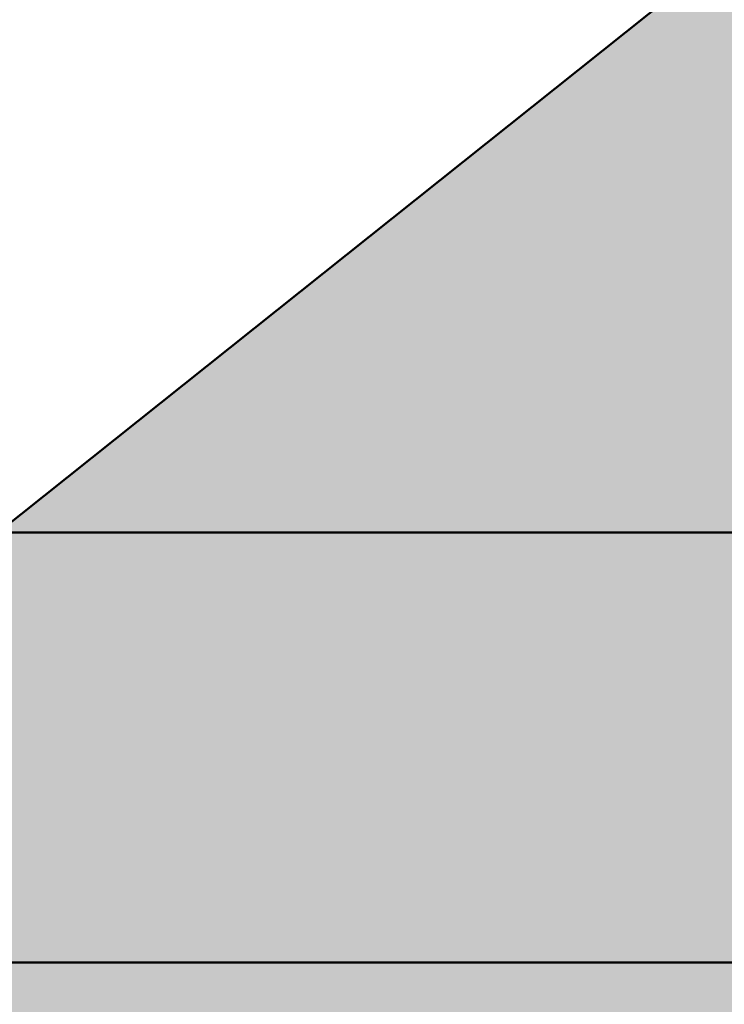
# Model space of a CAD drawing. Units: millimetres. Extents: x 0 to 2267, y 0 to 1823.
# Tile 18 of 256: x 1531 to 1548, y 1116 to 1139. Entities that reach past the tile are written whole.
import ezdxf

# ---------------------------------------------------------------- set-up
doc = ezdxf.new("R2010")
doc.units = ezdxf.units.MM
doc.header["$MEASUREMENT"] = 0
doc.layers.add('M-HATC', color=252, linetype='Continuous', lineweight=18)
doc.layers.add('M-OUTL', color=7, linetype='Continuous', lineweight=50)

msp = doc.modelspace()

# ---------------------------------------------------------------- hatches: boundary and pattern name
at = {"layer": 'M-HATC'}
h = msp.add_hatch(color=256, dxfattribs=at)
h.dxf.hatch_style = 1
h.paths.add_polyline_path([(2065.771, 1618.062, 0.236068), (2055.771, 1638.062), (1381.087, 1638.062, 0.236068), (1371.087, 1618.062), (1371.087, 1603.062), (2055.771, 1603.062), (2065.771, 1603.062)])
h.paths.add_polyline_path([(2062.772, 1550.296), (2062.772, 1560.296), (1374.086, 1560.296), (1374.086, 1550.296), (1374.086, 1540.296), (1384.086, 1540.296), (1389.086, 1540.296), (2062.772, 1540.296)])
h.paths.add_polyline_path([(1930.929, 1282.766), (1505.929, 1282.766), (1587.628, 1235.597, 0.131652), (1600.128, 1232.247), (1836.73, 1232.247, 0.131652), (1849.23, 1235.597)])
h.paths.add_polyline_path([(1930.929, 1117.417), (1905.929, 1117.417), (1505.929, 1117.417), (1505.929, 1077.417), (1930.929, 1077.417)])
h = msp.add_hatch(color=256, dxfattribs=at)
h.dxf.hatch_style = 1
h.paths.add_polyline_path([(2055.771, 1603.062), (1381.087, 1603.062), (1381.087, 1598.062), (2055.771, 1598.062)])
h.paths.add_polyline_path([(2055.771, 1598.062), (1381.087, 1598.062), (1381.087, 1593.062), (2055.771, 1593.062)])
h.paths.add_polyline_path([(2051.307, 1536.761), (1385.55, 1536.761), (1385.55, 1526.761), (1387.55, 1526.761), (1388.537, 1525.053), (1385.332, 1521.233), (1385.332, 1521.223), (2050.254, 1522.749), (2048.321, 1525.053), (2049.307, 1526.761), (2051.307, 1526.761)])
edge = h.paths.add_edge_path()
edge.add_arc((1847.535, 1379.149), 135, 222.60306, 222.89085, ccw=False)
edge.add_line((1748.166, 1287.766), (1683.092, 1287.766))
edge.add_arc((1583.724, 1379.149), 135, 317.10915, 317.39694, ccw=False)
edge.add_arc((1678.969, 1290.671), 5, 222.8909, 317.1091, ccw=False)
edge.add_arc((1774.213, 1379.149), 135, 222.60306, 222.89085, ccw=False)
edge.add_line((1674.845, 1287.766), (1609.771, 1287.766))
edge.add_arc((1510.403, 1379.149), 135, 317.10915, 317.39694, ccw=False)
edge.add_arc((1605.647, 1290.671), 5, 222.8909, 317.1091, ccw=False)
edge.add_arc((1700.892, 1379.149), 135, 222.60306, 222.89085, ccw=False)
edge.add_line((1601.524, 1287.766), (1536.45, 1287.766))
edge.add_arc((1437.081, 1379.149), 135, 317.10915, 317.39694, ccw=False)
edge.add_arc((1532.326, 1290.671), 5, 222.8909, 317.1091, ccw=False)
edge.add_arc((1627.571, 1379.149), 135, 222.60306, 222.89085, ccw=False)
edge.add_line((1528.203, 1287.766), (1505.929, 1287.766))
edge.add_spline(control_points=[(1505.929, 1287.766), (1504.262, 1287.766), (1504.262, 1282.766), (1505.929, 1282.766)], knot_values=[0, 0, 0, 0, 5, 5, 5, 5], degree=3, periodic=0)
edge.add_line((1505.929, 1282.766), (1930.929, 1282.766))
edge.add_spline(control_points=[(1930.929, 1282.766), (1932.596, 1282.766), (1932.596, 1287.766), (1930.929, 1287.766)], knot_values=[0, 0, 0, 0, 5, 5, 5, 5], degree=3, periodic=0)
edge.add_line((1930.929, 1287.766), (1903.056, 1287.766))
edge.add_arc((1803.688, 1379.149), 135, 317.10915, 317.39694, ccw=False)
edge.add_arc((1898.932, 1290.671), 5, 222.8909, 317.1091, ccw=False)
edge.add_arc((1994.177, 1379.149), 135, 222.60306, 222.89085, ccw=False)
edge.add_line((1894.809, 1287.766), (1829.735, 1287.766))
edge.add_arc((1730.366, 1379.149), 135, 317.10915, 317.39694, ccw=False)
edge.add_arc((1825.611, 1290.671), 5, 222.8909, 317.1091, ccw=False)
edge.add_arc((1920.856, 1379.149), 135, 222.60306, 222.89085, ccw=False)
edge.add_line((1821.487, 1287.766), (1756.413, 1287.766))
edge.add_arc((1657.045, 1379.149), 135, 317.10915, 317.39694, ccw=False)
edge.add_arc((1752.29, 1290.671), 5, 222.8909, 317.1091, ccw=False)
edge = h.paths.add_edge_path()
edge.add_spline(control_points=[(1843.429, 1227.247), (1845.096, 1227.247), (1845.096, 1232.247), (1843.429, 1232.247)], knot_values=[0, 0, 0, 0, 5, 5, 5, 5], degree=3, periodic=0)
edge.add_line((1843.429, 1232.247), (1593.429, 1232.247))
edge.add_spline(control_points=[(1593.429, 1232.247), (1591.762, 1232.247), (1591.762, 1227.247), (1593.429, 1227.247)], knot_values=[0, 0, 0, 0, 5, 5, 5, 5], degree=3, periodic=0)
edge.add_line((1593.429, 1227.247), (1843.429, 1227.247))
h.paths.add_polyline_path([(1905.929, 1127.417), (1530.929, 1127.417, 0.414214), (1520.929, 1117.417), (1530.929, 1117.417), (1915.929, 1117.417, 0.414214)])
edge = h.paths.add_edge_path()
edge.add_arc((1397.086, 1498.408), 12.73, 90.7821, 190.8787, ccw=False)
edge.add_line((1396.912, 1511.136), (1428.01, 1511.349))
edge.add_line((1428.01, 1511.349), (1433.01, 1511.349))
edge.add_line((1433.01, 1511.349), (1434.439, 1511.349))
edge.add_arc((1419.474, 1498.08), 20, 41.561, 74.0821)
edge.add_line((1424.959, 1517.314), (1399.935, 1517.256))
edge.add_spline(control_points=[(1399.931, 1517.256), (1399.884, 1517.213), (1399.833, 1517.169), (1399.777, 1517.124)], knot_values=[11.567499, 11.567499, 11.567499, 11.567499, 11.814249, 11.814249, 11.814249, 11.814249], degree=3, periodic=0)
edge.add_spline(control_points=[(1399.633, 1517.01), (1399.583, 1516.972), (1399.531, 1516.934), (1399.476, 1516.895)], knot_values=[11.167718, 11.167718, 11.167718, 11.167718, 11.365188, 11.365188, 11.365188, 11.365188], degree=3, periodic=0)
edge.add_spline(control_points=[(1399.34, 1516.8), (1399.151, 1516.672), (1398.938, 1516.538), (1398.704, 1516.399)], knot_values=[10.376405, 10.376405, 10.376405, 10.376405, 11.00994, 11.00994, 11.00994, 11.00994], degree=3, periodic=0)
edge.add_spline(control_points=[(1398.657, 1516.372), (1398.579, 1516.326), (1398.498, 1516.28), (1398.415, 1516.233)], knot_values=[10.125175, 10.125175, 10.125175, 10.125175, 10.334406, 10.334406, 10.334406, 10.334406], degree=3, periodic=0)
edge.add_spline(control_points=[(1398.264, 1516.149), (1398.196, 1516.111), (1398.126, 1516.073), (1398.055, 1516.035)], knot_values=[9.832246, 9.832246, 9.832246, 9.832246, 9.999658, 9.999658, 9.999658, 9.999658], degree=3, periodic=0)
edge.add_spline(control_points=[(1397.999, 1516.005), (1397.731, 1515.862), (1397.446, 1515.717), (1397.147, 1515.571)], knot_values=[9.161808, 9.161808, 9.161808, 9.161808, 9.787769, 9.787769, 9.787769, 9.787769], degree=3, periodic=0)
edge.add_spline(control_points=[(1397.147, 1515.571), (1396.842, 1515.423), (1396.522, 1515.274), (1396.191, 1515.126)], knot_values=[8.524455, 8.524455, 8.524455, 8.524455, 9.161808, 9.161808, 9.161808, 9.161808], degree=3, periodic=0)
edge.add_spline(control_points=[(1396.078, 1515.076), (1395.985, 1515.035), (1395.892, 1514.994), (1395.798, 1514.953)], knot_values=[8.275193, 8.275193, 8.275193, 8.275193, 8.451726, 8.451726, 8.451726, 8.451726], degree=3, periodic=0)
edge.add_spline(control_points=[(1395.602, 1514.869), (1395.5, 1514.826), (1395.397, 1514.782), (1395.293, 1514.739)], knot_values=[7.962917, 7.962917, 7.962917, 7.962917, 8.152764, 8.152764, 8.152764, 8.152764], degree=3, periodic=0)
edge.add_spline(control_points=[(1395.212, 1514.706), (1394.828, 1514.547), (1394.435, 1514.393), (1394.036, 1514.244)], knot_values=[7.21254, 7.21254, 7.21254, 7.21254, 7.913148, 7.913148, 7.913148, 7.913148], degree=3, periodic=0)
edge.add_spline(control_points=[(1394.036, 1514.244), (1393.708, 1514.121), (1393.375, 1514.003), (1393.043, 1513.889)], knot_values=[6.633733, 6.633733, 6.633733, 6.633733, 7.21254, 7.21254, 7.21254, 7.21254], degree=3, periodic=0)
edge.add_spline(control_points=[(1392.821, 1513.815), (1392.72, 1513.781), (1392.618, 1513.748), (1392.517, 1513.715)], knot_values=[6.328796, 6.328796, 6.328796, 6.328796, 6.505493, 6.505493, 6.505493, 6.505493], degree=3, periodic=0)
edge.add_spline(control_points=[(1392.517, 1513.715), (1392.319, 1513.652), (1392.121, 1513.59), (1391.924, 1513.531)], knot_values=[5.984605, 5.984605, 5.984605, 5.984605, 6.328796, 6.328796, 6.328796, 6.328796], degree=3, periodic=0)
edge.add_spline(control_points=[(1391.792, 1513.491), (1391.312, 1513.35), (1390.838, 1513.224), (1390.378, 1513.117)], knot_values=[5.066697, 5.066697, 5.066697, 5.066697, 5.907055, 5.907055, 5.907055, 5.907055], degree=3, periodic=0)
edge.add_spline(control_points=[(1390.378, 1513.117), (1390.18, 1513.071), (1389.984, 1513.028), (1389.791, 1512.99)], knot_values=[4.70367, 4.70367, 4.70367, 4.70367, 5.066695, 5.066695, 5.066695, 5.066695], degree=3, periodic=0)
edge.add_spline(control_points=[(1389.422, 1512.92), (1389.246, 1512.889), (1389.073, 1512.862), (1388.904, 1512.838)], knot_values=[4.130571, 4.130571, 4.130571, 4.130571, 4.469816, 4.469816, 4.469816, 4.469816], degree=3, periodic=0)
edge.add_spline(control_points=[(1388.904, 1512.838), (1388.591, 1512.795), (1388.291, 1512.764), (1388.007, 1512.749)], knot_values=[3.504031, 3.504031, 3.504031, 3.504031, 4.130571, 4.130571, 4.130571, 4.130571], degree=3, periodic=0)
edge.add_spline(control_points=[(1387.936, 1512.746), (1387.854, 1512.742), (1387.773, 1512.74), (1387.694, 1512.739)], knot_values=[3.268866, 3.268866, 3.268866, 3.268866, 3.451164, 3.451164, 3.451164, 3.451164], degree=3, periodic=0)
edge.add_spline(control_points=[(1387.335, 1512.744), (1387.208, 1512.75), (1387.085, 1512.76), (1386.967, 1512.774)], knot_values=[2.670686, 2.670686, 2.670686, 2.670686, 2.984, 2.984, 2.984, 2.984], degree=3, periodic=0)
edge.add_spline(control_points=[(1386.833, 1512.792), (1386.821, 1512.794), (1386.809, 1512.796), (1386.797, 1512.798)], knot_values=[2.516981, 2.516981, 2.516981, 2.516981, 2.549528, 2.549528, 2.549528, 2.549528], degree=3, periodic=0)
edge.add_spline(control_points=[(1386.453, 1512.873), (1386.426, 1512.881), (1386.399, 1512.889), (1386.373, 1512.897)], knot_values=[2.095869, 2.095869, 2.095869, 2.095869, 2.17941, 2.17941, 2.17941, 2.17941], degree=3, periodic=0)
edge.add_spline(control_points=[(1386.069, 1513.019), (1386.063, 1513.022), (1386.058, 1513.025), (1386.052, 1513.028)], knot_values=[1.72453, 1.72453, 1.72453, 1.72453, 1.745933, 1.745933, 1.745933, 1.745933], degree=3, periodic=0)
edge.add_arc((1399.474, 1498.08), 20, 131.8243, 180)
edge.add_arc((1630.334, 1505.548), 250.971, 181.70518, 236.42798)
edge.add_arc((1605.34, 1483.304), 218.782, 238.66083, 243.34961)
edge.add_arc((1647.091, 1510.359), 262.899, 183.12984, 237.85344, ccw=False)
h.paths.add_polyline_path([(1406.537, 1391.964, 0.149382), (1491.551, 1296.442, -0.129517)], flags=17)
edge = h.paths.add_edge_path()
edge.add_arc((2037.384, 1498.08), 20, 0, 48.2659)
edge.add_spline(control_points=[(2050.697, 1513.005), (2050.651, 1512.985), (2050.603, 1512.966), (2050.554, 1512.948)], knot_values=[1.835652, 1.835652, 1.835652, 1.835652, 2.000781, 2.000781, 2.000781, 2.000781], degree=3, periodic=0)
edge.add_spline(control_points=[(2050.462, 1512.917), (2050.479, 1512.922), (2050.496, 1512.928), (2050.513, 1512.934)], knot_values=[2.045477, 2.045477, 2.045477, 2.045477, 2.101389, 2.101389, 2.101389, 2.101389], degree=3, periodic=0)
edge.add_spline(control_points=[(2050.129, 1512.834), (2050.198, 1512.847), (2050.266, 1512.862), (2050.331, 1512.879)], knot_values=[2.237629, 2.237629, 2.237629, 2.237629, 2.435841, 2.435841, 2.435841, 2.435841], degree=3, periodic=0)
edge.add_spline(control_points=[(2050.095, 1512.828), (2050.106, 1512.83), (2050.118, 1512.832), (2050.129, 1512.834)], knot_values=[2.435841, 2.435841, 2.435841, 2.435841, 2.468321, 2.468321, 2.468321, 2.468321], degree=3, periodic=0)
edge.add_spline(control_points=[(2049.784, 1512.785), (2049.855, 1512.792), (2049.924, 1512.801), (2049.992, 1512.811)], knot_values=[2.563852, 2.563852, 2.563852, 2.563852, 2.748541, 2.748541, 2.748541, 2.748541], degree=3, periodic=0)
edge.add_spline(control_points=[(2049.405, 1512.762), (2049.536, 1512.765), (2049.663, 1512.773), (2049.784, 1512.785)], knot_values=[2.748541, 2.748541, 2.748541, 2.748541, 3.064882, 3.064882, 3.064882, 3.064882], degree=3, periodic=0)
edge.add_spline(control_points=[(2049.17, 1512.76), (2049.234, 1512.759), (2049.297, 1512.759), (2049.358, 1512.761)], knot_values=[3.102309, 3.102309, 3.102309, 3.102309, 3.2503, 3.2503, 3.2503, 3.2503], degree=3, periodic=0)
edge.add_spline(control_points=[(2048.857, 1512.769), (2048.964, 1512.764), (2049.068, 1512.761), (2049.17, 1512.76)], knot_values=[3.2503, 3.2503, 3.2503, 3.2503, 3.486069, 3.486069, 3.486069, 3.486069], degree=3, periodic=0)
edge.add_spline(control_points=[(2048.692, 1512.779), (2048.373, 1512.801), (2048.035, 1512.841), (2047.682, 1512.897)], knot_values=[3.606429, 3.606429, 3.606429, 3.606429, 4.2989, 4.2989, 4.2989, 4.2989], degree=3, periodic=0)
edge.add_spline(control_points=[(2047.682, 1512.897), (2047.546, 1512.919), (2047.408, 1512.942), (2047.268, 1512.969)], knot_values=[4.2989, 4.2989, 4.2989, 4.2989, 4.565769, 4.565769, 4.565769, 4.565769], degree=3, periodic=0)
edge.add_spline(control_points=[(2047.268, 1512.969), (2047.145, 1512.991), (2047.021, 1513.016), (2046.895, 1513.042)], knot_values=[4.565769, 4.565769, 4.565769, 4.565769, 4.799971, 4.799971, 4.799971, 4.799971], degree=3, periodic=0)
edge.add_spline(control_points=[(2046.895, 1513.042), (2046.529, 1513.119), (2046.151, 1513.209), (2045.768, 1513.311)], knot_values=[4.799971, 4.799971, 4.799971, 4.799971, 5.483718, 5.483718, 5.483718, 5.483718], degree=3, periodic=0)
edge.add_spline(control_points=[(2045.768, 1513.311), (2045.372, 1513.415), (2044.97, 1513.532), (2044.566, 1513.659)], knot_values=[5.483718, 5.483718, 5.483718, 5.483718, 6.187866, 6.187866, 6.187866, 6.187866], degree=3, periodic=0)
edge.add_spline(control_points=[(2044.566, 1513.659), (2044.415, 1513.706), (2044.263, 1513.755), (2044.112, 1513.805)], knot_values=[6.187866, 6.187866, 6.187866, 6.187866, 6.451551, 6.451551, 6.451551, 6.451551], degree=3, periodic=0)
edge.add_spline(control_points=[(2044.112, 1513.805), (2043.997, 1513.843), (2043.882, 1513.881), (2043.767, 1513.92)], knot_values=[6.451551, 6.451551, 6.451551, 6.451551, 6.651434, 6.651434, 6.651434, 6.651434], degree=3, periodic=0)
edge.add_spline(control_points=[(2043.767, 1513.92), (2043.372, 1514.055), (2042.977, 1514.198), (2042.589, 1514.346)], knot_values=[6.651434, 6.651434, 6.651434, 6.651434, 7.338879, 7.338879, 7.338879, 7.338879], degree=3, periodic=0)
edge.add_spline(control_points=[(2042.589, 1514.346), (2042.164, 1514.507), (2041.746, 1514.675), (2041.341, 1514.846)], knot_values=[7.338879, 7.338879, 7.338879, 7.338879, 8.089209, 8.089209, 8.089209, 8.089209], degree=3, periodic=0)
edge.add_spline(control_points=[(2041.341, 1514.846), (2041.103, 1514.946), (2040.869, 1515.048), (2040.64, 1515.15)], knot_values=[8.089209, 8.089209, 8.089209, 8.089209, 8.529587, 8.529587, 8.529587, 8.529587], degree=3, periodic=0)
edge.add_spline(control_points=[(2040.51, 1515.209), (2040.082, 1515.402), (2039.675, 1515.597), (2039.295, 1515.789)], knot_values=[8.613818, 8.613818, 8.613818, 8.613818, 9.44571, 9.44571, 9.44571, 9.44571], degree=3, periodic=0)
edge.add_spline(control_points=[(2039.295, 1515.789), (2039.062, 1515.907), (2038.839, 1516.025), (2038.629, 1516.14)], knot_values=[9.44571, 9.44571, 9.44571, 9.44571, 9.956404, 9.956404, 9.956404, 9.956404], degree=3, periodic=0)
edge.add_spline(control_points=[(2038.629, 1516.14), (2038.519, 1516.2), (2038.412, 1516.26), (2038.309, 1516.319)], knot_values=[9.956404, 9.956404, 9.956404, 9.956404, 10.223542, 10.223542, 10.223542, 10.223542], degree=3, periodic=0)
edge.add_spline(control_points=[(2038.309, 1516.319), (2038.214, 1516.374), (2038.122, 1516.428), (2038.033, 1516.481)], knot_values=[10.223542, 10.223542, 10.223542, 10.223542, 10.47051, 10.47051, 10.47051, 10.47051], degree=3, periodic=0)
edge.add_spline(control_points=[(2038.033, 1516.481), (2037.786, 1516.63), (2037.564, 1516.773), (2037.372, 1516.909)], knot_values=[10.47051, 10.47051, 10.47051, 10.47051, 11.15767, 11.15767, 11.15767, 11.15767], degree=3, periodic=0)
edge.add_spline(control_points=[(2037.372, 1516.909), (2037.279, 1516.975), (2037.193, 1517.04), (2037.114, 1517.102)], knot_values=[11.15767, 11.15767, 11.15767, 11.15767, 11.49227, 11.49227, 11.49227, 11.49227], degree=3, periodic=0)
edge.add_spline(control_points=[(2036.856, 1517.326), (2036.915, 1517.269), (2036.981, 1517.21), (2037.056, 1517.149)], knot_values=[11.577341, 11.577341, 11.577341, 11.577341, 11.91035, 11.91035, 11.91035, 11.91035], degree=3, periodic=0)
edge.add_spline(control_points=[(2036.807, 1517.375), (2036.823, 1517.359), (2036.839, 1517.342), (2036.856, 1517.326)], knot_values=[11.91035, 11.91035, 11.91035, 11.91035, 12.007402, 12.007402, 12.007402, 12.007402], degree=3, periodic=0)
edge.add_spline(control_points=[(2036.702, 1517.494), (2036.71, 1517.483), (2036.72, 1517.472), (2036.729, 1517.461)], knot_values=[12.184155, 12.184155, 12.184155, 12.184155, 12.255409, 12.255409, 12.255409, 12.255409], degree=3, periodic=0)
edge.add_spline(control_points=[(2036.616, 1517.621), (2036.62, 1517.613), (2036.624, 1517.606), (2036.629, 1517.598)], knot_values=[12.487913, 12.487913, 12.487913, 12.487913, 12.541035, 12.541035, 12.541035, 12.541035], degree=3, periodic=0)
edge.add_spline(control_points=[(2036.563, 1517.786), (2036.564, 1517.779), (2036.564, 1517.773), (2036.565, 1517.766)], knot_values=[12.911761, 12.911761, 12.911761, 12.911761, 12.968286, 12.968286, 12.968286, 12.968286], degree=3, periodic=0)
edge.add_spline(control_points=[(2036.617, 1517.93), (2036.612, 1517.926), (2036.609, 1517.921), (2036.605, 1517.916)], knot_values=[13.382527, 13.382527, 13.382527, 13.382527, 13.433791, 13.433791, 13.433791, 13.433791], degree=3, periodic=0)
edge.add_spline(control_points=[(2036.749, 1518.017), (2036.736, 1518.012), (2036.724, 1518.006), (2036.712, 1518)], knot_values=[13.726299, 13.726299, 13.726299, 13.726299, 13.809928, 13.809928, 13.809928, 13.809928], degree=3, periodic=0)
edge.add_spline(control_points=[(2036.86, 1518.053), (2036.839, 1518.047), (2036.818, 1518.042), (2036.799, 1518.035)], knot_values=[13.910887, 13.910887, 13.910887, 13.910887, 14.02153, 14.02153, 14.02153, 14.02153], degree=3, periodic=0)
edge.add_line((2036.964, 1518.08), (2032.384, 1518.08))
edge.add_line((2032.384, 1518.08), (2027.384, 1518.08))
edge.add_line((2027.384, 1518.08), (2022.384, 1518.08))
edge.add_line((2022.384, 1518.08), (2017.384, 1518.08))
edge.add_arc((2017.384, 1498.08), 20, 90, 138.439)
edge.add_line((2002.419, 1511.349), (2003.848, 1511.349))
edge.add_line((2003.848, 1511.349), (2008.848, 1511.349))
edge.add_line((2008.848, 1511.349), (2039.772, 1511.138))
edge.add_arc((2039.772, 1498.408), 12.73, -10.8787, 90, ccw=False)
edge.add_arc((1789.767, 1510.359), 262.899, 302.14656, 356.87016, ccw=False)
edge.add_arc((1831.518, 1483.304), 218.782, 296.65039, 301.33917)
edge.add_arc((1806.524, 1505.548), 250.971, 303.57202, 358.29482)
h.paths.add_polyline_path([(2030.321, 1391.964, -0.129517), (1945.307, 1296.442, 0.149382)], flags=17)
edge = h.paths.add_edge_path()
edge.add_spline(control_points=[(2037.246, 1518.082), (2037.29, 1518.081), (2037.336, 1518.08), (2037.384, 1518.08)], knot_values=[0.000012, 0.000012, 0.000012, 0.000012, 0.144754, 0.144754, 0.144754, 0.144754], degree=3, periodic=0)
edge.add_line((2037.336, 1518.08), (2037.01, 1518.08))
edge.add_spline(control_points=[(2037.01, 1518.08), (2036.982, 1518.077), (2036.956, 1518.073), (2036.931, 1518.068)], knot_values=[14.13465, 14.13465, 14.13465, 14.13465, 14.247197, 14.247197, 14.247197, 14.247197], degree=3, periodic=0)
edge.add_spline(control_points=[(2036.931, 1518.068), (2036.928, 1518.067), (2036.924, 1518.067), (2036.921, 1518.066)], knot_values=[14.118315, 14.118315, 14.118315, 14.118315, 14.13465, 14.13465, 14.13465, 14.13465], degree=3, periodic=0)
edge.add_spline(control_points=[(2036.921, 1518.066), (2036.912, 1518.064), (2036.903, 1518.063), (2036.895, 1518.061)], knot_values=[14.078086, 14.078086, 14.078086, 14.078086, 14.118315, 14.118315, 14.118315, 14.118315], degree=3, periodic=0)
edge.add_spline(control_points=[(2036.895, 1518.061), (2036.883, 1518.058), (2036.872, 1518.056), (2036.86, 1518.053)], knot_values=[14.02153, 14.02153, 14.02153, 14.02153, 14.078086, 14.078086, 14.078086, 14.078086], degree=3, periodic=0)
edge.add_spline(control_points=[(2036.86, 1518.053), (2036.839, 1518.047), (2036.818, 1518.042), (2036.799, 1518.035)], knot_values=[13.910887, 13.910887, 13.910887, 13.910887, 14.02153, 14.02153, 14.02153, 14.02153], degree=3, periodic=0)
edge.add_spline(control_points=[(2036.799, 1518.035), (2036.798, 1518.035), (2036.797, 1518.035), (2036.797, 1518.035)], knot_values=[13.906906, 13.906906, 13.906906, 13.906906, 13.910887, 13.910887, 13.910887, 13.910887], degree=3, periodic=0)
edge.add_spline(control_points=[(2036.797, 1518.035), (2036.788, 1518.032), (2036.78, 1518.029), (2036.772, 1518.026)], knot_values=[13.857826, 13.857826, 13.857826, 13.857826, 13.906906, 13.906906, 13.906906, 13.906906], degree=3, periodic=0)
edge.add_spline(control_points=[(2036.772, 1518.026), (2036.764, 1518.023), (2036.756, 1518.02), (2036.749, 1518.017)], knot_values=[13.809928, 13.809928, 13.809928, 13.809928, 13.857826, 13.857826, 13.857826, 13.857826], degree=3, periodic=0)
edge.add_spline(control_points=[(2036.749, 1518.017), (2036.736, 1518.012), (2036.724, 1518.006), (2036.712, 1518)], knot_values=[13.726299, 13.726299, 13.726299, 13.726299, 13.809928, 13.809928, 13.809928, 13.809928], degree=3, periodic=0)
edge.add_spline(control_points=[(2036.712, 1518), (2036.712, 1518), (2036.712, 1518), (2036.711, 1518)], knot_values=[13.723993, 13.723993, 13.723993, 13.723993, 13.726299, 13.726299, 13.726299, 13.726299], degree=3, periodic=0)
edge.add_spline(control_points=[(2036.711, 1518), (2036.706, 1517.997), (2036.701, 1517.994), (2036.696, 1517.992)], knot_values=[13.686536, 13.686536, 13.686536, 13.686536, 13.723993, 13.723993, 13.723993, 13.723993], degree=3, periodic=0)
edge.add_spline(control_points=[(2036.696, 1517.992), (2036.692, 1517.989), (2036.687, 1517.987), (2036.683, 1517.984)], knot_values=[13.651251, 13.651251, 13.651251, 13.651251, 13.686536, 13.686536, 13.686536, 13.686536], degree=3, periodic=0)
edge.add_spline(control_points=[(2036.683, 1517.984), (2036.676, 1517.98), (2036.67, 1517.976), (2036.664, 1517.971)], knot_values=[13.596804, 13.596804, 13.596804, 13.596804, 13.651251, 13.651251, 13.651251, 13.651251], degree=3, periodic=0)
edge.add_spline(control_points=[(2036.664, 1517.971), (2036.664, 1517.971), (2036.663, 1517.971), (2036.663, 1517.971)], knot_values=[13.593956, 13.593956, 13.593956, 13.593956, 13.596804, 13.596804, 13.596804, 13.596804], degree=3, periodic=0)
edge.add_spline(control_points=[(2036.663, 1517.971), (2036.66, 1517.969), (2036.658, 1517.967), (2036.655, 1517.965)], knot_values=[13.570322, 13.570322, 13.570322, 13.570322, 13.593956, 13.593956, 13.593956, 13.593956], degree=3, periodic=0)
edge.add_spline(control_points=[(2036.655, 1517.965), (2036.653, 1517.963), (2036.65, 1517.961), (2036.647, 1517.959)], knot_values=[13.545477, 13.545477, 13.545477, 13.545477, 13.570322, 13.570322, 13.570322, 13.570322], degree=3, periodic=0)
edge.add_spline(control_points=[(2036.647, 1517.959), (2036.647, 1517.959), (2036.647, 1517.959), (2036.647, 1517.959)], knot_values=[13.543931, 13.543931, 13.543931, 13.543931, 13.545477, 13.545477, 13.545477, 13.545477], degree=3, periodic=0)
edge.add_spline(control_points=[(2036.647, 1517.959), (2036.641, 1517.954), (2036.636, 1517.949), (2036.631, 1517.945)], knot_values=[13.488237, 13.488237, 13.488237, 13.488237, 13.543931, 13.543931, 13.543931, 13.543931], degree=3, periodic=0)
edge.add_spline(control_points=[(2036.631, 1517.945), (2036.628, 1517.942), (2036.626, 1517.94), (2036.623, 1517.937)], knot_values=[13.460307, 13.460307, 13.460307, 13.460307, 13.488237, 13.488237, 13.488237, 13.488237], degree=3, periodic=0)
edge.add_spline(control_points=[(2036.623, 1517.937), (2036.622, 1517.936), (2036.62, 1517.934), (2036.618, 1517.932)], knot_values=[13.439712, 13.439712, 13.439712, 13.439712, 13.460307, 13.460307, 13.460307, 13.460307], degree=3, periodic=0)
edge.add_spline(control_points=[(2036.618, 1517.932), (2036.618, 1517.931), (2036.617, 1517.931), (2036.617, 1517.93)], knot_values=[13.433791, 13.433791, 13.433791, 13.433791, 13.439712, 13.439712, 13.439712, 13.439712], degree=3, periodic=0)
edge.add_spline(control_points=[(2036.617, 1517.93), (2036.612, 1517.926), (2036.609, 1517.921), (2036.605, 1517.916)], knot_values=[13.382527, 13.382527, 13.382527, 13.382527, 13.433791, 13.433791, 13.433791, 13.433791], degree=3, periodic=0)
edge.add_spline(control_points=[(2036.605, 1517.916), (2036.603, 1517.913), (2036.6, 1517.91), (2036.598, 1517.907)], knot_values=[13.350017, 13.350017, 13.350017, 13.350017, 13.382527, 13.382527, 13.382527, 13.382527], degree=3, periodic=0)
edge.add_spline(control_points=[(2036.598, 1517.907), (2036.597, 1517.906), (2036.596, 1517.904), (2036.595, 1517.903)], knot_values=[13.333922, 13.333922, 13.333922, 13.333922, 13.350017, 13.350017, 13.350017, 13.350017], degree=3, periodic=0)
edge.add_spline(control_points=[(2036.595, 1517.903), (2036.595, 1517.902), (2036.594, 1517.901), (2036.593, 1517.9)], knot_values=[13.323828, 13.323828, 13.323828, 13.323828, 13.333922, 13.333922, 13.333922, 13.333922], degree=3, periodic=0)
edge.add_spline(control_points=[(2036.593, 1517.9), (2036.59, 1517.895), (2036.588, 1517.891), (2036.585, 1517.886)], knot_values=[13.277545, 13.277545, 13.277545, 13.277545, 13.323828, 13.323828, 13.323828, 13.323828], degree=3, periodic=0)
edge.add_spline(control_points=[(2036.585, 1517.886), (2036.584, 1517.883), (2036.582, 1517.879), (2036.58, 1517.875)], knot_values=[13.240119, 13.240119, 13.240119, 13.240119, 13.277545, 13.277545, 13.277545, 13.277545], degree=3, periodic=0)
edge.add_spline(control_points=[(2036.58, 1517.875), (2036.58, 1517.874), (2036.579, 1517.873), (2036.578, 1517.872)], knot_values=[13.228211, 13.228211, 13.228211, 13.228211, 13.240119, 13.240119, 13.240119, 13.240119], degree=3, periodic=0)
edge.add_spline(control_points=[(2036.578, 1517.872), (2036.578, 1517.87), (2036.577, 1517.869), (2036.577, 1517.868)], knot_values=[13.215717, 13.215717, 13.215717, 13.215717, 13.228211, 13.228211, 13.228211, 13.228211], degree=3, periodic=0)
edge.add_spline(control_points=[(2036.577, 1517.868), (2036.575, 1517.864), (2036.574, 1517.86), (2036.573, 1517.857)], knot_values=[13.179847, 13.179847, 13.179847, 13.179847, 13.215717, 13.215717, 13.215717, 13.215717], degree=3, periodic=0)
edge.add_spline(control_points=[(2036.573, 1517.857), (2036.571, 1517.851), (2036.57, 1517.846), (2036.569, 1517.841)], knot_values=[13.132017, 13.132017, 13.132017, 13.132017, 13.179847, 13.179847, 13.179847, 13.179847], degree=3, periodic=0)
edge.add_spline(control_points=[(2036.569, 1517.841), (2036.568, 1517.84), (2036.568, 1517.839), (2036.568, 1517.838)], knot_values=[13.122482, 13.122482, 13.122482, 13.122482, 13.132017, 13.132017, 13.132017, 13.132017], degree=3, periodic=0)
edge.add_spline(control_points=[(2036.568, 1517.838), (2036.568, 1517.836), (2036.567, 1517.835), (2036.567, 1517.833)], knot_values=[13.105592, 13.105592, 13.105592, 13.105592, 13.122482, 13.122482, 13.122482, 13.122482], degree=3, periodic=0)
edge.add_spline(control_points=[(2036.567, 1517.833), (2036.566, 1517.829), (2036.566, 1517.826), (2036.565, 1517.822)], knot_values=[13.074063, 13.074063, 13.074063, 13.074063, 13.105592, 13.105592, 13.105592, 13.105592], degree=3, periodic=0)
edge.add_spline(control_points=[(2036.565, 1517.822), (2036.565, 1517.822), (2036.565, 1517.822), (2036.565, 1517.822)], knot_values=[13.074043, 13.074043, 13.074043, 13.074043, 13.074063, 13.074063, 13.074063, 13.074063], degree=3, periodic=0)
edge.add_spline(control_points=[(2036.565, 1517.822), (2036.564, 1517.816), (2036.564, 1517.811), (2036.564, 1517.805)], knot_values=[13.021884, 13.021884, 13.021884, 13.021884, 13.074043, 13.074043, 13.074043, 13.074043], degree=3, periodic=0)
edge.add_spline(control_points=[(2036.564, 1517.805), (2036.564, 1517.804), (2036.564, 1517.803), (2036.564, 1517.803)], knot_values=[13.01674, 13.01674, 13.01674, 13.01674, 13.021884, 13.021884, 13.021884, 13.021884], degree=3, periodic=0)
edge.add_spline(control_points=[(2036.564, 1517.803), (2036.563, 1517.801), (2036.563, 1517.798), (2036.563, 1517.796)], knot_values=[12.996438, 12.996438, 12.996438, 12.996438, 13.01674, 13.01674, 13.01674, 13.01674], degree=3, periodic=0)
edge.add_spline(control_points=[(2036.563, 1517.796), (2036.563, 1517.793), (2036.563, 1517.789), (2036.563, 1517.786)], knot_values=[12.968286, 12.968286, 12.968286, 12.968286, 12.996438, 12.996438, 12.996438, 12.996438], degree=3, periodic=0)
edge.add_spline(control_points=[(2036.563, 1517.786), (2036.564, 1517.779), (2036.564, 1517.773), (2036.565, 1517.766)], knot_values=[12.911761, 12.911761, 12.911761, 12.911761, 12.968286, 12.968286, 12.968286, 12.968286], degree=3, periodic=0)
edge.add_spline(control_points=[(2036.565, 1517.766), (2036.565, 1517.766), (2036.565, 1517.766), (2036.565, 1517.766)], knot_values=[12.911017, 12.911017, 12.911017, 12.911017, 12.911761, 12.911761, 12.911761, 12.911761], degree=3, periodic=0)
edge.add_spline(control_points=[(2036.565, 1517.766), (2036.565, 1517.762), (2036.566, 1517.759), (2036.566, 1517.756)], knot_values=[12.88528, 12.88528, 12.88528, 12.88528, 12.911017, 12.911017, 12.911017, 12.911017], degree=3, periodic=0)
edge.add_spline(control_points=[(2036.566, 1517.756), (2036.567, 1517.753), (2036.567, 1517.751), (2036.568, 1517.748)], knot_values=[12.862519, 12.862519, 12.862519, 12.862519, 12.88528, 12.88528, 12.88528, 12.88528], degree=3, periodic=0)
edge.add_spline(control_points=[(2036.568, 1517.748), (2036.568, 1517.747), (2036.568, 1517.747), (2036.568, 1517.746)], knot_values=[12.858885, 12.858885, 12.858885, 12.858885, 12.862519, 12.862519, 12.862519, 12.862519], degree=3, periodic=0)
edge.add_spline(control_points=[(2036.568, 1517.746), (2036.569, 1517.74), (2036.571, 1517.733), (2036.572, 1517.726)], knot_values=[12.8053, 12.8053, 12.8053, 12.8053, 12.858885, 12.858885, 12.858885, 12.858885], degree=3, periodic=0)
edge.add_spline(control_points=[(2036.572, 1517.726), (2036.573, 1517.723), (2036.574, 1517.719), (2036.576, 1517.715)], knot_values=[12.775176, 12.775176, 12.775176, 12.775176, 12.8053, 12.8053, 12.8053, 12.8053], degree=3, periodic=0)
edge.add_spline(control_points=[(2036.576, 1517.715), (2036.576, 1517.713), (2036.577, 1517.71), (2036.578, 1517.708)], knot_values=[12.756759, 12.756759, 12.756759, 12.756759, 12.775176, 12.775176, 12.775176, 12.775176], degree=3, periodic=0)
edge.add_spline(control_points=[(2036.578, 1517.708), (2036.578, 1517.707), (2036.578, 1517.706), (2036.579, 1517.705)], knot_values=[12.748742, 12.748742, 12.748742, 12.748742, 12.756759, 12.756759, 12.756759, 12.756759], degree=3, periodic=0)
edge.add_spline(control_points=[(2036.579, 1517.705), (2036.581, 1517.698), (2036.583, 1517.692), (2036.586, 1517.685)], knot_values=[12.69959, 12.69959, 12.69959, 12.69959, 12.748742, 12.748742, 12.748742, 12.748742], degree=3, periodic=0)
edge.add_spline(control_points=[(2036.586, 1517.685), (2036.588, 1517.68), (2036.59, 1517.675), (2036.592, 1517.669)], knot_values=[12.659038, 12.659038, 12.659038, 12.659038, 12.69959, 12.69959, 12.69959, 12.69959], degree=3, periodic=0)
edge.add_spline(control_points=[(2036.592, 1517.669), (2036.594, 1517.665), (2036.596, 1517.66), (2036.598, 1517.656)], knot_values=[12.626806, 12.626806, 12.626806, 12.626806, 12.659038, 12.659038, 12.659038, 12.659038], degree=3, periodic=0)
edge.add_spline(control_points=[(2036.598, 1517.656), (2036.598, 1517.655), (2036.599, 1517.654), (2036.599, 1517.653)], knot_values=[12.619394, 12.619394, 12.619394, 12.619394, 12.626806, 12.626806, 12.626806, 12.626806], degree=3, periodic=0)
edge.add_spline(control_points=[(2036.599, 1517.653), (2036.604, 1517.642), (2036.61, 1517.632), (2036.616, 1517.621)], knot_values=[12.541039, 12.541039, 12.541039, 12.541039, 12.619394, 12.619394, 12.619394, 12.619394], degree=3, periodic=0)
edge.add_spline(control_points=[(2036.616, 1517.621), (2036.616, 1517.621), (2036.616, 1517.621), (2036.616, 1517.621)], knot_values=[12.541035, 12.541035, 12.541035, 12.541035, 12.541039, 12.541039, 12.541039, 12.541039], degree=3, periodic=0)
edge.add_spline(control_points=[(2036.616, 1517.621), (2036.62, 1517.613), (2036.624, 1517.606), (2036.629, 1517.598)], knot_values=[12.487913, 12.487913, 12.487913, 12.487913, 12.541035, 12.541035, 12.541035, 12.541035], degree=3, periodic=0)
edge.add_spline(control_points=[(2036.629, 1517.598), (2036.633, 1517.592), (2036.637, 1517.585), (2036.641, 1517.579)], knot_values=[12.443982, 12.443982, 12.443982, 12.443982, 12.487913, 12.487913, 12.487913, 12.487913], degree=3, periodic=0)
edge.add_spline(control_points=[(2036.641, 1517.579), (2036.641, 1517.578), (2036.642, 1517.576), (2036.643, 1517.575)], knot_values=[12.434996, 12.434996, 12.434996, 12.434996, 12.443982, 12.443982, 12.443982, 12.443982], degree=3, periodic=0)
edge.add_spline(control_points=[(2036.643, 1517.575), (2036.653, 1517.56), (2036.664, 1517.544), (2036.676, 1517.528)], knot_values=[12.329647, 12.329647, 12.329647, 12.329647, 12.434996, 12.434996, 12.434996, 12.434996], degree=3, periodic=0)
edge.add_spline(control_points=[(2036.676, 1517.528), (2036.684, 1517.517), (2036.693, 1517.505), (2036.702, 1517.494)], knot_values=[12.255409, 12.255409, 12.255409, 12.255409, 12.329647, 12.329647, 12.329647, 12.329647], degree=3, periodic=0)
edge.add_spline(control_points=[(2036.702, 1517.494), (2036.71, 1517.483), (2036.72, 1517.472), (2036.729, 1517.461)], knot_values=[12.184155, 12.184155, 12.184155, 12.184155, 12.255409, 12.255409, 12.255409, 12.255409], degree=3, periodic=0)
edge.add_spline(control_points=[(2036.729, 1517.461), (2036.744, 1517.444), (2036.759, 1517.426), (2036.775, 1517.409)], knot_values=[12.075961, 12.075961, 12.075961, 12.075961, 12.184155, 12.184155, 12.184155, 12.184155], degree=3, periodic=0)
edge.add_spline(control_points=[(2036.775, 1517.409), (2036.776, 1517.407), (2036.777, 1517.406), (2036.778, 1517.405)], knot_values=[12.069502, 12.069502, 12.069502, 12.069502, 12.075961, 12.075961, 12.075961, 12.075961], degree=3, periodic=0)
edge.add_spline(control_points=[(2036.778, 1517.405), (2036.788, 1517.395), (2036.797, 1517.385), (2036.807, 1517.375)], knot_values=[12.007402, 12.007402, 12.007402, 12.007402, 12.069502, 12.069502, 12.069502, 12.069502], degree=3, periodic=0)
edge.add_spline(control_points=[(2036.807, 1517.375), (2036.823, 1517.359), (2036.839, 1517.342), (2036.856, 1517.326)], knot_values=[11.91035, 11.91035, 11.91035, 11.91035, 12.007402, 12.007402, 12.007402, 12.007402], degree=3, periodic=0)
edge.add_spline(control_points=[(2036.856, 1517.326), (2036.915, 1517.269), (2036.981, 1517.21), (2037.056, 1517.149)], knot_values=[11.577341, 11.577341, 11.577341, 11.577341, 11.91035, 11.91035, 11.91035, 11.91035], degree=3, periodic=0)
edge.add_spline(control_points=[(2037.056, 1517.149), (2037.075, 1517.134), (2037.094, 1517.118), (2037.114, 1517.102)], knot_values=[11.49227, 11.49227, 11.49227, 11.49227, 11.577341, 11.577341, 11.577341, 11.577341], degree=3, periodic=0)
edge.add_spline(control_points=[(2037.114, 1517.102), (2037.193, 1517.04), (2037.279, 1516.975), (2037.372, 1516.909)], knot_values=[11.15767, 11.15767, 11.15767, 11.15767, 11.49227, 11.49227, 11.49227, 11.49227], degree=3, periodic=0)
edge.add_spline(control_points=[(2037.372, 1516.909), (2037.564, 1516.773), (2037.786, 1516.63), (2038.033, 1516.481)], knot_values=[10.47051, 10.47051, 10.47051, 10.47051, 11.15767, 11.15767, 11.15767, 11.15767], degree=3, periodic=0)
edge.add_spline(control_points=[(2038.033, 1516.481), (2038.122, 1516.428), (2038.214, 1516.374), (2038.309, 1516.319)], knot_values=[10.223542, 10.223542, 10.223542, 10.223542, 10.47051, 10.47051, 10.47051, 10.47051], degree=3, periodic=0)
edge.add_spline(control_points=[(2038.309, 1516.319), (2038.412, 1516.26), (2038.519, 1516.2), (2038.629, 1516.14)], knot_values=[9.956404, 9.956404, 9.956404, 9.956404, 10.223542, 10.223542, 10.223542, 10.223542], degree=3, periodic=0)
edge.add_spline(control_points=[(2038.629, 1516.14), (2038.839, 1516.025), (2039.062, 1515.907), (2039.295, 1515.789)], knot_values=[9.44571, 9.44571, 9.44571, 9.44571, 9.956404, 9.956404, 9.956404, 9.956404], degree=3, periodic=0)
edge.add_spline(control_points=[(2039.295, 1515.789), (2039.675, 1515.597), (2040.082, 1515.402), (2040.51, 1515.209)], knot_values=[8.613818, 8.613818, 8.613818, 8.613818, 9.44571, 9.44571, 9.44571, 9.44571], degree=3, periodic=0)
edge.add_spline(control_points=[(2040.51, 1515.209), (2040.553, 1515.189), (2040.597, 1515.17), (2040.64, 1515.15)], knot_values=[8.529587, 8.529587, 8.529587, 8.529587, 8.613818, 8.613818, 8.613818, 8.613818], degree=3, periodic=0)
edge.add_spline(control_points=[(2040.64, 1515.15), (2040.869, 1515.048), (2041.103, 1514.946), (2041.341, 1514.846)], knot_values=[8.089209, 8.089209, 8.089209, 8.089209, 8.529587, 8.529587, 8.529587, 8.529587], degree=3, periodic=0)
edge.add_spline(control_points=[(2041.341, 1514.846), (2041.746, 1514.675), (2042.164, 1514.507), (2042.589, 1514.346)], knot_values=[7.338879, 7.338879, 7.338879, 7.338879, 8.089209, 8.089209, 8.089209, 8.089209], degree=3, periodic=0)
edge.add_spline(control_points=[(2042.589, 1514.346), (2042.977, 1514.198), (2043.372, 1514.055), (2043.767, 1513.92)], knot_values=[6.651434, 6.651434, 6.651434, 6.651434, 7.338879, 7.338879, 7.338879, 7.338879], degree=3, periodic=0)
edge.add_spline(control_points=[(2043.767, 1513.92), (2043.882, 1513.881), (2043.997, 1513.843), (2044.112, 1513.805)], knot_values=[6.451551, 6.451551, 6.451551, 6.451551, 6.651434, 6.651434, 6.651434, 6.651434], degree=3, periodic=0)
edge.add_spline(control_points=[(2044.112, 1513.805), (2044.263, 1513.755), (2044.415, 1513.706), (2044.566, 1513.659)], knot_values=[6.187866, 6.187866, 6.187866, 6.187866, 6.451551, 6.451551, 6.451551, 6.451551], degree=3, periodic=0)
edge.add_spline(control_points=[(2044.566, 1513.659), (2044.97, 1513.532), (2045.372, 1513.415), (2045.768, 1513.311)], knot_values=[5.483718, 5.483718, 5.483718, 5.483718, 6.187866, 6.187866, 6.187866, 6.187866], degree=3, periodic=0)
edge.add_spline(control_points=[(2045.768, 1513.311), (2046.151, 1513.209), (2046.529, 1513.119), (2046.895, 1513.042)], knot_values=[4.799971, 4.799971, 4.799971, 4.799971, 5.483718, 5.483718, 5.483718, 5.483718], degree=3, periodic=0)
edge.add_spline(control_points=[(2046.895, 1513.042), (2047.021, 1513.016), (2047.145, 1512.991), (2047.268, 1512.969)], knot_values=[4.565769, 4.565769, 4.565769, 4.565769, 4.799971, 4.799971, 4.799971, 4.799971], degree=3, periodic=0)
edge.add_spline(control_points=[(2047.268, 1512.969), (2047.408, 1512.942), (2047.546, 1512.919), (2047.682, 1512.897)], knot_values=[4.2989, 4.2989, 4.2989, 4.2989, 4.565769, 4.565769, 4.565769, 4.565769], degree=3, periodic=0)
edge.add_spline(control_points=[(2047.682, 1512.897), (2048.035, 1512.841), (2048.373, 1512.801), (2048.692, 1512.779)], knot_values=[3.606429, 3.606429, 3.606429, 3.606429, 4.2989, 4.2989, 4.2989, 4.2989], degree=3, periodic=0)
edge.add_spline(control_points=[(2048.692, 1512.779), (2048.748, 1512.775), (2048.803, 1512.772), (2048.857, 1512.769)], knot_values=[3.486069, 3.486069, 3.486069, 3.486069, 3.606429, 3.606429, 3.606429, 3.606429], degree=3, periodic=0)
edge.add_spline(control_points=[(2048.857, 1512.769), (2048.964, 1512.764), (2049.068, 1512.761), (2049.17, 1512.76)], knot_values=[3.2503, 3.2503, 3.2503, 3.2503, 3.486069, 3.486069, 3.486069, 3.486069], degree=3, periodic=0)
edge.add_spline(control_points=[(2049.17, 1512.76), (2049.234, 1512.759), (2049.297, 1512.759), (2049.358, 1512.761)], knot_values=[3.102309, 3.102309, 3.102309, 3.102309, 3.2503, 3.2503, 3.2503, 3.2503], degree=3, periodic=0)
edge.add_spline(control_points=[(2049.358, 1512.761), (2049.374, 1512.761), (2049.39, 1512.761), (2049.405, 1512.762)], knot_values=[3.064882, 3.064882, 3.064882, 3.064882, 3.102309, 3.102309, 3.102309, 3.102309], degree=3, periodic=0)
edge.add_spline(control_points=[(2049.405, 1512.762), (2049.536, 1512.765), (2049.663, 1512.773), (2049.784, 1512.785)], knot_values=[2.748541, 2.748541, 2.748541, 2.748541, 3.064882, 3.064882, 3.064882, 3.064882], degree=3, periodic=0)
edge.add_spline(control_points=[(2049.784, 1512.785), (2049.855, 1512.792), (2049.924, 1512.801), (2049.992, 1512.811)], knot_values=[2.563852, 2.563852, 2.563852, 2.563852, 2.748541, 2.748541, 2.748541, 2.748541], degree=3, periodic=0)
edge.add_spline(control_points=[(2049.992, 1512.811), (2050.026, 1512.816), (2050.061, 1512.822), (2050.095, 1512.828)], knot_values=[2.468321, 2.468321, 2.468321, 2.468321, 2.563852, 2.563852, 2.563852, 2.563852], degree=3, periodic=0)
edge.add_spline(control_points=[(2050.095, 1512.828), (2050.106, 1512.83), (2050.118, 1512.832), (2050.129, 1512.834)], knot_values=[2.435841, 2.435841, 2.435841, 2.435841, 2.468321, 2.468321, 2.468321, 2.468321], degree=3, periodic=0)
edge.add_spline(control_points=[(2050.129, 1512.834), (2050.198, 1512.847), (2050.266, 1512.862), (2050.331, 1512.879)], knot_values=[2.237629, 2.237629, 2.237629, 2.237629, 2.435841, 2.435841, 2.435841, 2.435841], degree=3, periodic=0)
edge.add_spline(control_points=[(2050.331, 1512.879), (2050.375, 1512.891), (2050.419, 1512.903), (2050.462, 1512.917)], knot_values=[2.101389, 2.101389, 2.101389, 2.101389, 2.237629, 2.237629, 2.237629, 2.237629], degree=3, periodic=0)
edge.add_spline(control_points=[(2050.462, 1512.917), (2050.479, 1512.922), (2050.496, 1512.928), (2050.513, 1512.934)], knot_values=[2.045477, 2.045477, 2.045477, 2.045477, 2.101389, 2.101389, 2.101389, 2.101389], degree=3, periodic=0)
edge.add_spline(control_points=[(2050.513, 1512.934), (2050.527, 1512.938), (2050.54, 1512.943), (2050.554, 1512.948)], knot_values=[2.000781, 2.000781, 2.000781, 2.000781, 2.045477, 2.045477, 2.045477, 2.045477], degree=3, periodic=0)
edge.add_spline(control_points=[(2050.554, 1512.948), (2050.603, 1512.966), (2050.651, 1512.985), (2050.697, 1513.005)], knot_values=[1.835652, 1.835652, 1.835652, 1.835652, 2.000781, 2.000781, 2.000781, 2.000781], degree=3, periodic=0)
edge.add_arc((2037.384, 1498.08), 20, 48.2659, 90.1299)
edge = h.paths.add_edge_path(flags=16)
edge.add_spline(control_points=[(1386.139, 1512.986), (1388.92, 1511.739), (1398.039, 1515.519), (1399.931, 1517.256)], knot_values=[1.831046, 1.831046, 1.831046, 1.831046, 11.814249, 11.814249, 11.814249, 11.814249], degree=3, periodic=0)
edge.add_line((1399.931, 1517.256), (1393.743, 1517.242))
edge.add_arc((1399.474, 1498.08), 20, 106.6501, 131.8173)
h = msp.add_hatch(color=256, dxfattribs=at)
h.dxf.hatch_style = 1
h.paths.add_polyline_path([(2042.889, 1580.18), (2055.771, 1593.062), (1381.087, 1593.062), (1393.969, 1580.18), (1374.086, 1560.296), (2062.772, 1560.296)])
h.paths.add_polyline_path([(1843.429, 1201.33), (1843.429, 1227.247), (1593.429, 1227.247), (1593.429, 1201.33, -0.228274), (1574.599, 1162.235), (1530.929, 1127.417), (1905.929, 1127.417), (1862.259, 1162.235, -0.228274)])

# ---------------------------------------------------------------- linework, layer by layer
at = {"layer": 'M-OUTL'}
for p, q in [((1574.599, 1162.235), (1530.929, 1127.417)), ((1530.929, 1127.417), (1905.929, 1127.417)), ((1505.929, 1117.417), (1930.929, 1117.417))]:
    msp.add_line(p, q, dxfattribs=at)

doc.saveas('drawing.dxf')
